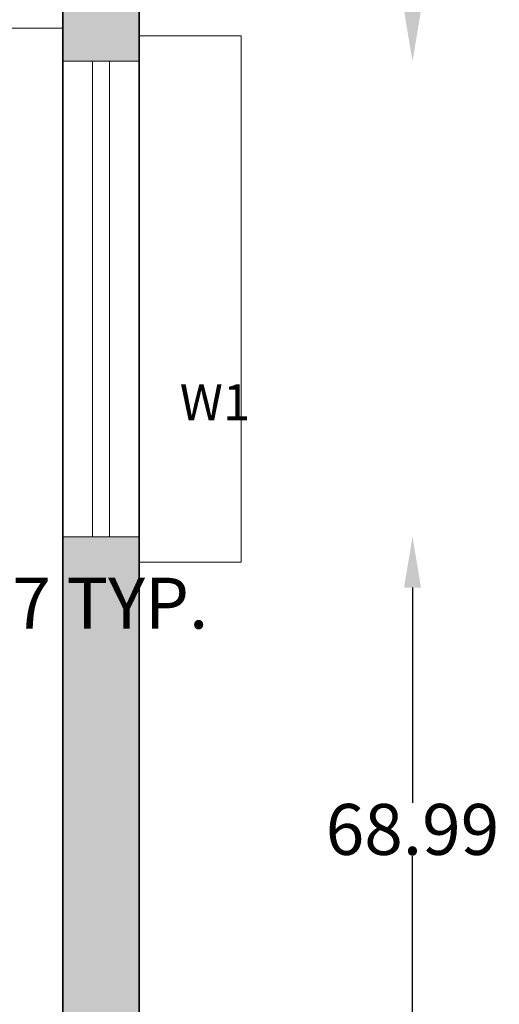
# Model space of a CAD drawing. Units: inches. Extents: x 1994 to 3075, y 3517 to 3950.
# Tile 57 of 58: x 3019 to 3075, y 3621 to 3737. Entities that reach past the tile are written whole.
import ezdxf

# ---------------------------------------------------------------- set-up
doc = ezdxf.new("R2010")
doc.units = ezdxf.units.IN
for name, color, linetype, lineweight in [('A-ANNO-DIMS', 2, 'Continuous', 18), ('A-ANNO-TEXT', 7, 'Continuous', 18), ('A-FLOR-CASE', 8, 'Continuous', 18), ('A-GLAZ', 4, 'Continuous', 18), ('A-GLAZ-PROJ', 4, 'Continuous', 18), ('A-WALL', 7, 'Continuous', 35), ('A-WALL-PATT', 252, 'Continuous', 13)]:
    doc.layers.add(name, color=color, linetype=linetype, lineweight=lineweight)
doc.styles.get("Standard").update_dxf_attribs({"font": 'arial.ttf'})
doc.dimstyles.get("Standard").update_dxf_attribs({"dimtxt": 6, "dimasz": 6, "dimexe": 0.18, "dimexo": 0.0625, "dimgap": 0.09, "dimtad": 0, "dimtih": 1, "dimtoh": 1, "dimdec": 4, "dimzin": 0, "dimdsep": 46, "dimlunit": 4, "dimtxsty": 'Standard', "dimcen": 0.09, "dimse1": 1, "dimse2": 1, "dimadec": 0, "dimazin": 0, "dimtfac": 1, "dimtdec": 4, "dimtofl": 0, "dimtmove": 0, "dimatfit": 3, "dimfxl": 1, "dimtolj": 1, "dimtzin": 0, "dimarcsym": 0})

# ---------------------------------------------------------------- blocks, each defined once
blk = doc.blocks.new('WINDOW-56IN-SASH')
for p, q in [((56.01, 9), (0, 9)), ((0, 5.5), (56.01, 5.5)), ((0, 3.5), (56.01, 3.5)), ((0, 0), (56.01, 0))]:
    blk.add_line(p, q)
blk = doc.blocks.new('WINDOW-HOOD-62IN')
for p, q in [((0, 59.01), (0, 62.01)), ((0, 62.01), (12, 62.01)), ((0, 0), (0, 59.01)), ((12, 0), (0, 0))]:
    blk.add_line(p, q)
blk = doc.blocks.new('*D25')
at = {"layer": 'A-ANNO-DIMS', "color": 0, "lineweight": -2, "transparency": 16777216}
for p, q in [((2943.67, 3662.28), (2943.67, 3668.28)), ((2943.67, 3668.28), (2949.67, 3668.28)), ((2943.67, 3651.18), (2943.67, 3656.28))]:
    blk.add_line(p, q, dxfattribs=at)
at = {"layer": 'A-ANNO-DIMS', "color": 0, "transparency": 16777216}
for points in [[(2942.67, 3656.28), (2944.67, 3656.28), (2943.67, 3662.28)], [(2942.67, 3651.18), (2944.67, 3651.18), (2943.67, 3645.18)]]:
    blk.add_solid(points, dxfattribs=at)
at = {"layer": 'Defpoints', "color": 0, "transparency": 16777216}
for p in [(2941.1, 3662.28), (2943.67, 3662.28), (2941.1, 3645.18)]:
    blk.add_point(p, dxfattribs=at)
at = {"layer": 'A-ANNO-DIMS', "color": 0, "transparency": 16777216, "insert": (2997.3, 3668.28), "char_height": 6, "attachment_point": 5}
blk.add_mtext('\\A1;LOUNGE CHAIR 17 TYP.', dxfattribs=at)
blk = doc.blocks.new('*D37')
at = {"layer": 'A-ANNO-DIMS', "color": 0, "lineweight": -2, "transparency": 16777216}
for p, q in [((3065.27, 3670.11), (3065.27, 3644.77)), ((3065.27, 3613.13), (3065.27, 3638.47))]:
    blk.add_line(p, q, dxfattribs=at)
at = {"layer": 'A-ANNO-DIMS', "color": 0, "transparency": 16777216}
for points in [[(3064.27, 3670.11), (3066.27, 3670.11), (3065.27, 3676.11)], [(3064.27, 3613.13), (3066.27, 3613.13), (3065.27, 3607.13)]]:
    blk.add_solid(points, dxfattribs=at)
at = {"layer": 'Defpoints', "color": 0, "transparency": 16777216}
for p in [(3033.07, 3676.11), (3065.27, 3676.11), (3033.07, 3607.13)]:
    blk.add_point(p, dxfattribs=at)
at = {"layer": 'A-ANNO-DIMS', "color": 0, "transparency": 16777216, "insert": (3065.27, 3641.62), "char_height": 6, "attachment_point": 5}
blk.add_mtext('\\A1;68.99', dxfattribs=at)
blk = doc.blocks.new('*D38')
at = {"layer": 'A-ANNO-DIMS', "color": 0, "lineweight": -2, "transparency": 16777216}
for p, q in [((3065.27, 3799.41), (3065.27, 3771.92)), ((3065.27, 3738.12), (3065.27, 3765.61))]:
    blk.add_line(p, q, dxfattribs=at)
at = {"layer": 'A-ANNO-DIMS', "color": 0, "transparency": 16777216}
for points in [[(3064.27, 3799.41), (3066.27, 3799.41), (3065.27, 3805.41)], [(3064.27, 3738.12), (3066.27, 3738.12), (3065.27, 3732.12)]]:
    blk.add_solid(points, dxfattribs=at)
at = {"layer": 'Defpoints', "color": 0, "transparency": 16777216}
for p in [(3033.07, 3805.41), (3065.27, 3805.41), (3033.07, 3732.12)]:
    blk.add_point(p, dxfattribs=at)
at = {"layer": 'A-ANNO-DIMS', "color": 0, "transparency": 16777216, "insert": (3065.27, 3768.77), "char_height": 6, "attachment_point": 5}
blk.add_mtext('\\A1;73.28', dxfattribs=at)

msp = doc.modelspace()

# ---------------------------------------------------------------- hatches: boundary and pattern name
at = {"layer": 'A-WALL-PATT'}
h = msp.add_hatch(color=256, dxfattribs=at)
h.dxf.hatch_style = 1
h.paths.add_polyline_path([(2678.072, 3755.1269), (2669.072, 3755.1269), (2669.072, 3718.5523), (2678.072, 3718.5523)])
h.paths.add_polyline_path([(2807.072, 3761.1269), (2678.072, 3761.1269), (2678.072, 3755.1269), (2807.072, 3755.1269)])
h.paths.add_polyline_path([(2678.072, 3812.7371), (2669.072, 3812.7371), (2669.072, 3809.7371), (2669.072, 3764.1269), (2678.072, 3764.1269)])
h.paths.add_polyline_path([(2678.072, 3905.1269), (2669.072, 3905.1269), (2669.072, 3868.7491), (2678.072, 3868.7491)])
h.paths.add_polyline_path([(2723.826, 3914.1269), (2720.826, 3914.1269), (2678.072, 3914.1269), (2678.072, 3905.1269), (2723.826, 3905.1269)])
h.paths.add_polyline_path([(2807.072, 3914.1269), (2779.838, 3914.1269), (2779.838, 3905.1269), (2807.072, 3905.1269)])
h.paths.add_polyline_path([(2837.6979, 3914.1269), (2834.6979, 3914.1269), (2820.9062, 3914.1269), (2816.072, 3914.1269), (2816.072, 3905.1269), (2837.6979, 3905.1269)])
h.paths.add_polyline_path([(2885.9096, 3914.1269), (2869.71, 3914.1269), (2869.71, 3905.1269), (2876.9183, 3905.1269), (2885.9096, 3905.1269)])
h.paths.add_polyline_path([(2933.6904, 3914.1269), (2930.6904, 3914.1269), (2894.9096, 3914.1269), (2894.9096, 3905.1269), (2933.6904, 3905.1269)])
h.paths.add_polyline_path([(3024.072, 3914.1269), (2989.7025, 3914.1269), (2989.7025, 3905.1269), (3024.072, 3905.1269)])
h.paths.add_polyline_path([(3033.072, 3905.1269), (3024.072, 3905.1269), (3024.072, 3861.4192), (3033.072, 3861.4192)])
h.paths.add_polyline_path([(3033.072, 3805.4072), (3024.072, 3805.4072), (3024.072, 3764.1269), (3033.072, 3764.1269)])
h.paths.add_polyline_path([(3033.072, 3755.1269), (3024.072, 3755.1269), (3024.072, 3732.1247), (3033.072, 3732.1247), (3033.072, 3735.1247)])
h.paths.add_polyline_path([(3024.072, 3761.1269), (2895.072, 3761.1269), (2895.072, 3755.1269), (3024.072, 3755.1269)])
h.paths.add_polyline_path([(3033.072, 3676.1126), (3024.072, 3676.1126), (3024.072, 3616.1269), (3033.072, 3616.1269)])
h.paths.add_polyline_path([(3024.072, 3613.1269), (2959.4908, 3613.1269), (2959.4908, 3607.1269), (3024.072, 3607.1269)])
h.paths.add_polyline_path([(2914.1254, 3613.1269), (2894.9096, 3613.1269), (2894.9096, 3607.1269), (2914.1254, 3607.1269)])
h.paths.add_polyline_path([(2885.9096, 3613.1269), (2852.072, 3613.1269), (2852.072, 3607.1269), (2885.9096, 3607.1269)])
h.paths.add_polyline_path([(2822.072, 3613.1269), (2810.072, 3613.1269), (2810.072, 3559.1269), (2816.072, 3559.1269), (2816.072, 3607.1269), (2822.072, 3607.1269)])
h.paths.add_polyline_path([(2933.072, 3607.1269), (2924.072, 3607.1269), (2924.072, 3550.1269), (2892.072, 3550.1269), (2816.072, 3550.1269), (2810.072, 3550.1269), (2810.072, 3541.1269), (2892.072, 3541.1269), (2933.072, 3541.1269)])
h.paths.add_polyline_path([(2807.072, 3559.1269), (2678.072, 3559.1269), (2678.072, 3550.1269), (2807.072, 3550.1269)])
h.paths.add_polyline_path([(2678.072, 3655.1269), (2669.072, 3655.1269), (2669.072, 3559.1269), (2678.072, 3559.1269)])
h.paths.add_polyline_path([(2678.072, 3686.5403), (2669.072, 3686.5403), (2669.072, 3664.1269), (2678.072, 3664.1269)])
h.paths.add_polyline_path([(2807.072, 3661.1269), (2678.072, 3661.1269), (2678.072, 3655.1269), (2807.072, 3655.1269)])
h.paths.add_polyline_path([(2816.072, 3755.1269), (2810.072, 3755.1269), (2810.072, 3703.1269), (2816.072, 3703.1269)])
h.paths.add_polyline_path([(2816.072, 3905.1269), (2810.072, 3905.1269), (2810.072, 3803.1269), (2816.072, 3803.1269), (2816.072, 3815.1269)])
h.paths.add_polyline_path([(2886.072, 3821.1269), (2852.072, 3821.1269), (2852.072, 3815.1269), (2886.072, 3815.1269)])
h.paths.add_polyline_path([(2822.072, 3821.1269), (2816.072, 3821.1269), (2816.072, 3815.1269), (2822.072, 3815.1269)])
h.paths.add_polyline_path([(2892.072, 3905.1269), (2886.072, 3905.1269), (2886.072, 3803.1269), (2892.072, 3803.1269)])

# ---------------------------------------------------------------- linework, layer by layer
at = {"layer": 'A-FLOR-CASE'}
msp.add_line((2984.6205, 3736.0298), (3024.072, 3736.0298), dxfattribs=at)
at = {"layer": 'A-GLAZ'}
for p, q in [((3033.072, 3732.1247), (3024.072, 3732.1247)), ((3024.072, 3676.1126), (3033.072, 3676.1126))]:
    msp.add_line(p, q, dxfattribs=at)
at = {"layer": 'A-GLAZ-PROJ'}
msp.add_line((3033.072, 3732.1247), (3033.072, 3735.1247), dxfattribs=at)
at = {"layer": 'A-WALL'}
for p, q in [((3033.072, 3914.1269), (3033.072, 3607.1269)), ((3024.072, 3905.1269), (3024.072, 3607.1269))]:
    msp.add_line(p, q, dxfattribs=at)

# ---------------------------------------------------------------- block references
at = {"layer": 'A-GLAZ', "rotation": 89.9999999999982}
msp.add_blockref('WINDOW-56IN-SASH', (3033.0719, 3676.1126), dxfattribs=at)
at = {"layer": 'A-GLAZ-PROJ', "rotation": 180}
msp.add_blockref('WINDOW-HOOD-62IN', (3045.0721, 3735.1247), dxfattribs=at)

# ---------------------------------------------------------------- texts
at = {"layer": 'A-ANNO-TEXT', "insert": (3037.8551, 3694.0809), "char_height": 4.24528, "attachment_point": 1}
msp.add_mtext_dynamic_manual_height_columns('W1', width=102.693633, gutter_width=21.2264, heights=[0], dxfattribs=at)

# ---------------------------------------------------------------- dimensions: what is measured, and where the dimension line sits
at = {"layer": 'A-ANNO-DIMS'}
for base, p1, p2, picture, middle in [((3065.272, 3805.4072), (3033.072, 3732.1247), (3033.072, 3805.4072), '*D38', (3065.272, 3768.7659)), ((3065.272, 3676.1126), (3033.072, 3607.1269), (3033.072, 3676.1126), '*D37', (3065.272, 3641.6197))]:
    dim = msp.add_linear_dim(base=base, p1=p1, p2=p2, angle=90, dimstyle='Standard', override={"dimdec": 2, "dimlfac": 1, "dimrnd": 0, "dimzin": 0, "dimdsep": 46, "dimlunit": 2}, dxfattribs=at)
    dim.commit()
    dim.dimension.update_dxf_attribs({"geometry": picture, "text_midpoint": middle})
dim = msp.add_linear_dim(base=(2943.6687, 3662.2807), p1=(2941.1031, 3645.1769), p2=(2941.1031, 3662.2807), angle=90, text='LOUNGE CHAIR <> TYP.', dimstyle='Standard', override={"dimdec": 0, "dimlfac": 1, "dimrnd": 0, "dimzin": 0, "dimdsep": 46, "dimlunit": 2}, dxfattribs=at)
dim.commit()
dim.dimension.update_dxf_attribs({"geometry": '*D25', "text_midpoint": (2997.2962, 3668.2807)})

doc.saveas('drawing.dxf')
